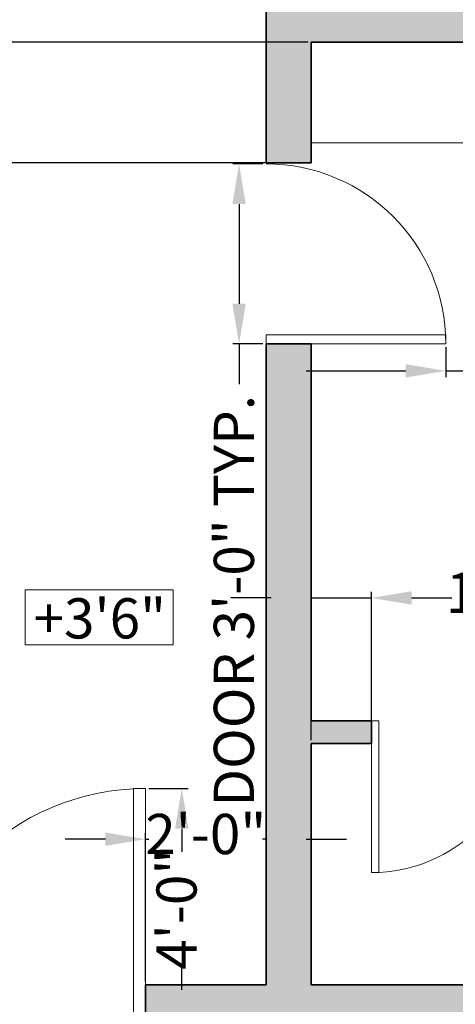
# Model space of a CAD drawing. Units: inches. Extents: x 2408 to 5087, y 2429 to 5085.
# Tile 8 of 12: x 2636 to 2723, y 2619 to 2815. Entities that reach past the tile are written whole.
import ezdxf

# ---------------------------------------------------------------- set-up
doc = ezdxf.new("R2010")
doc.units = ezdxf.units.IN
for name, color, linetype, lineweight in [('A-ANNO-DIMS', 2, 'Continuous', 18), ('A-ANNO-SYMB', 6, 'Continuous', 18), ('A-DOOR', 3, 'Continuous', 18), ('A-FLOR-CASE', 8, 'Continuous', 18), ('A-WALL', 7, 'Continuous', 35), ('A-WALL-PATT', 252, 'Continuous', 13)]:
    doc.layers.add(name, color=color, linetype=linetype, lineweight=lineweight)
doc.styles.get("Standard").update_dxf_attribs({"font": 'arial.ttf'})
doc.dimstyles.new('ISO-25', dxfattribs={"dimtxt": 8, "dimasz": 8, "dimexe": 1.25, "dimexo": 0.625, "dimtad": 0, "dimdec": 1, "dimlunit": 4, "dimtxsty": 'Standard', "dimcen": 2.5, "dimadec": 0, "dimazin": 0, "dimtfac": 1, "dimtdec": 1, "dimtmove": 0, "dimatfit": 3, "dimfxl": 1, "dimarcsym": 0})

# ---------------------------------------------------------------- blocks, each defined once
blk = doc.blocks.new('door')
blk.add_lwpolyline([(2353.25, 2862.23), (2353.25, 2898.06), (2351.47, 2898.06), (2351.47, 2862.23), (2353.25, 2862.23)])
blk.add_arc((2353.25, 2862.23), 35.83, 90, 180)
blk = doc.blocks.new('LEVEL-TAG-FRAME')
blk.add_line((29.47, 11), (29.47, 0))
blk.add_lwpolyline([(29.47, 0), (0, 0), (0, 11), (29.47, 11)])
blk = doc.blocks.new('*D27')
at = {"layer": 'A-ANNO-DIMS', "color": 0, "lineweight": -2, "transparency": 16777216}
for p, q in [((2612.36, 2568.68), (2612.36, 2576.68)), ((2608.98, 2568.68), (2613.61, 2568.68)), ((2612.36, 2550.04), (2612.36, 2560.68)), ((2608.98, 2542.04), (2613.61, 2542.04))]:
    blk.add_line(p, q, dxfattribs=at)
at = {"layer": 'A-ANNO-DIMS', "color": 0, "transparency": 16777216}
for points in [[(2611.02, 2560.68), (2613.69, 2560.68), (2612.36, 2568.68)], [(2611.02, 2550.04), (2613.69, 2550.04), (2612.36, 2542.04)]]:
    blk.add_solid(points, dxfattribs=at)
at = {"layer": 'Defpoints', "color": 0, "transparency": 16777216}
for p in [(2608.36, 2568.68), (2612.36, 2568.68), (2608.36, 2542.04)]:
    blk.add_point(p, dxfattribs=at)
at = {"layer": 'A-ANNO-DIMS', "color": 0, "transparency": 16777216, "insert": (2612.36, 2631.3), "char_height": 8, "attachment_point": 5, "rotation": 90}
blk.add_mtext('PAVER 2\'-2 1/2" TYP.', dxfattribs=at)
blk = doc.blocks.new('*D37')
at = {"layer": 'A-ANNO-DIMS', "color": 0, "lineweight": -2, "transparency": 16777216}
for p, q in [((2684.87, 2785.87), (2678.87, 2785.87)), ((2680.12, 2777.87), (2680.12, 2758.05)), ((2684.87, 2750.05), (2678.87, 2750.05)), ((2680.12, 2750.05), (2680.12, 2742.05))]:
    blk.add_line(p, q, dxfattribs=at)
at = {"layer": 'A-ANNO-DIMS', "color": 0, "transparency": 16777216}
for points in [[(2678.79, 2777.87), (2681.45, 2777.87), (2680.12, 2785.87)], [(2678.79, 2758.05), (2681.45, 2758.05), (2680.12, 2750.05)]]:
    blk.add_solid(points, dxfattribs=at)
at = {"layer": 'Defpoints', "color": 0, "transparency": 16777216}
for p in [(2685.49, 2785.87), (2680.12, 2750.05), (2685.49, 2750.05)]:
    blk.add_point(p, dxfattribs=at)
at = {"layer": 'A-ANNO-DIMS', "color": 0, "transparency": 16777216, "insert": (2680.12, 2698.93), "char_height": 8, "attachment_point": 5, "rotation": 90}
blk.add_mtext('DOOR 3\'-0" TYP.', dxfattribs=at)
blk = doc.blocks.new('*D38')
at = {"layer": 'A-ANNO-DIMS', "color": 0, "lineweight": -2, "transparency": 16777216}
for p, q in [((2685.49, 2749.43), (2685.49, 2743.43)), ((2721.31, 2749.43), (2721.31, 2743.43)), ((2693.49, 2744.68), (2713.31, 2744.68)), ((2721.31, 2744.68), (2729.31, 2744.68))]:
    blk.add_line(p, q, dxfattribs=at)
at = {"layer": 'A-ANNO-DIMS', "color": 0, "transparency": 16777216}
for points in [[(2693.49, 2746.02), (2693.49, 2743.35), (2685.49, 2744.68)], [(2713.31, 2746.02), (2713.31, 2743.35), (2721.31, 2744.68)]]:
    blk.add_solid(points, dxfattribs=at)
at = {"layer": 'Defpoints', "color": 0, "transparency": 16777216}
for p in [(2685.49, 2750.05), (2721.31, 2750.05), (2721.31, 2744.68)]:
    blk.add_point(p, dxfattribs=at)
at = {"layer": 'A-ANNO-DIMS', "color": 0, "transparency": 16777216, "insert": (2754.31, 2744.68), "char_height": 8, "attachment_point": 5}
blk.add_mtext('3\'-0" TYP.', dxfattribs=at)
blk = doc.blocks.new('*D40')
at = {"layer": 'A-ANNO-DIMS', "color": 0, "lineweight": -2, "transparency": 16777216}
for p, q in [((2662.12, 2661.59), (2669.95, 2661.59)), ((2668.7, 2653.59), (2668.7, 2648.99)), ((2668.7, 2621.55), (2668.7, 2626.15)), ((2662.12, 2613.55), (2669.95, 2613.55))]:
    blk.add_line(p, q, dxfattribs=at)
at = {"layer": 'A-ANNO-DIMS', "color": 0, "transparency": 16777216}
for points in [[(2667.37, 2653.59), (2670.03, 2653.59), (2668.7, 2661.59)], [(2667.37, 2621.55), (2670.03, 2621.55), (2668.7, 2613.55)]]:
    blk.add_solid(points, dxfattribs=at)
at = {"layer": 'Defpoints', "color": 0, "transparency": 16777216}
for p in [(2661.49, 2661.59), (2668.7, 2661.59), (2661.49, 2613.55)]:
    blk.add_point(p, dxfattribs=at)
at = {"layer": 'A-ANNO-DIMS', "color": 0, "transparency": 16777216, "insert": (2668.7, 2637.57), "char_height": 8, "attachment_point": 5, "rotation": 90}
blk.add_mtext('4\'-0"', dxfattribs=at)
blk = doc.blocks.new('*D75')
at = {"layer": 'A-ANNO-DIMS', "color": 0, "lineweight": -2, "transparency": 16777216}
for p, q in [((2661.49, 2623.18), (2661.49, 2652.75)), ((2685.49, 2623.18), (2685.49, 2652.75)), ((2653.49, 2651.5), (2645.49, 2651.5)), ((2661.49, 2651.5), (2662.17, 2651.5)), ((2685.49, 2651.5), (2684.82, 2651.5)), ((2693.49, 2651.5), (2701.49, 2651.5))]:
    blk.add_line(p, q, dxfattribs=at)
at = {"layer": 'A-ANNO-DIMS', "color": 0, "transparency": 16777216}
for points in [[(2653.49, 2652.84), (2653.49, 2650.17), (2661.49, 2651.5)], [(2693.49, 2652.84), (2693.49, 2650.17), (2685.49, 2651.5)]]:
    blk.add_solid(points, dxfattribs=at)
at = {"layer": 'Defpoints', "color": 0, "transparency": 16777216}
for p in [(2685.49, 2651.5), (2661.49, 2622.55), (2685.49, 2622.55)]:
    blk.add_point(p, dxfattribs=at)
at = {"layer": 'A-ANNO-DIMS', "color": 0, "transparency": 16777216, "insert": (2673.49, 2651.5), "char_height": 8, "attachment_point": 5}
blk.add_mtext('2\'-0"', dxfattribs=at)
blk = doc.blocks.new('*D79')
at = {"layer": 'A-ANNO-DIMS', "color": 0, "lineweight": -2, "transparency": 16777216}
for p, q in [((2432.93, 2818.05), (2432.93, 2826.05)), ((2693.87, 2810.05), (2431.68, 2810.05)), ((2432.93, 2810.05), (2432.93, 2809.38)), ((2693.87, 2786.05), (2431.68, 2786.05)), ((2432.93, 2786.05), (2432.93, 2786.73)), ((2432.93, 2778.05), (2432.93, 2770.05))]:
    blk.add_line(p, q, dxfattribs=at)
at = {"layer": 'A-ANNO-DIMS', "color": 0, "transparency": 16777216}
for points in [[(2431.59, 2818.05), (2434.26, 2818.05), (2432.93, 2810.05)], [(2431.59, 2778.05), (2434.26, 2778.05), (2432.93, 2786.05)]]:
    blk.add_solid(points, dxfattribs=at)
at = {"layer": 'Defpoints', "color": 0, "transparency": 16777216}
for p in [(2432.93, 2810.05), (2694.49, 2810.05), (2694.49, 2786.05)]:
    blk.add_point(p, dxfattribs=at)
at = {"layer": 'A-ANNO-DIMS', "color": 0, "transparency": 16777216, "insert": (2432.93, 2798.05), "char_height": 8, "attachment_point": 5, "rotation": 90}
blk.add_mtext('2\'-0"', dxfattribs=at)
blk = doc.blocks.new('*D80')
at = {"layer": 'A-ANNO-DIMS', "color": 0, "lineweight": -2, "transparency": 16777216}
for p, q in [((2694.49, 2671.18), (2694.49, 2700.75)), ((2706.49, 2671.18), (2706.49, 2700.75)), ((2686.49, 2699.5), (2678.49, 2699.5)), ((2694.49, 2699.5), (2706.49, 2699.5)), ((2714.49, 2699.5), (2722.49, 2699.5))]:
    blk.add_line(p, q, dxfattribs=at)
at = {"layer": 'A-ANNO-DIMS', "color": 0, "transparency": 16777216}
for points in [[(2686.49, 2700.84), (2686.49, 2698.17), (2694.49, 2699.5)], [(2714.49, 2700.84), (2714.49, 2698.17), (2706.49, 2699.5)]]:
    blk.add_solid(points, dxfattribs=at)
at = {"layer": 'Defpoints', "color": 0, "transparency": 16777216}
for p in [(2706.49, 2699.5), (2694.49, 2670.55), (2706.49, 2670.55)]:
    blk.add_point(p, dxfattribs=at)
at = {"layer": 'A-ANNO-DIMS', "color": 0, "transparency": 16777216, "insert": (2733.38, 2699.5), "char_height": 8, "attachment_point": 5}
blk.add_mtext('1\'-0"', dxfattribs=at)

msp = doc.modelspace()

# ---------------------------------------------------------------- hatches: boundary and pattern name
at = {"layer": 'A-WALL-PATT'}
h = msp.add_hatch(color=256, dxfattribs=at)
h.dxf.hatch_style = 1
h.paths.add_polyline_path([(2493.49, 2613.55), (2523.49, 2613.55), (2523.49, 2622.55), (2493.49, 2622.55), (2493.49, 2714.8), (2484.49, 2714.8), (2484.49, 2497.75), (2493.49, 2497.75)])
h.paths.add_polyline_path([(2613.49, 2615.42), (2613.49, 2622.55), (2583.49, 2622.55), (2583.49, 2613.55), (2613.46, 2613.55, -0.009707)])
h.paths.add_polyline_path([(2823.49, 2634.55), (2814.49, 2634.55), (2814.49, 2622.55), (2694.49, 2622.55), (2694.49, 2670.55), (2706.49, 2670.55), (2706.49, 2675.05), (2694.49, 2675.05), (2694.49, 2750.05), (2685.49, 2750.05), (2685.49, 2622.55), (2661.49, 2622.55), (2661.49, 2613.55), (2814.49, 2613.55), (2814.49, 2522.05), (2688.49, 2522.05), (2688.49, 2513.05), (2823.49, 2513.05)])
h.paths.add_polyline_path([(2823.49, 2837.05), (2814.49, 2837.05), (2814.49, 2819.05), (2685.49, 2819.05), (2685.49, 2786.05), (2694.49, 2786.05), (2694.49, 2810.05), (2814.49, 2810.05), (2814.49, 2772.55), (2823.49, 2772.55)])
h.paths.add_polyline_path([(2694.49, 2964.55), (2595.49, 2964.55), (2595.49, 3008.05), (2601.49, 3008.05), (2601.49, 3017.05), (2484.49, 3017.05), (2484.49, 2972.05), (2493.49, 2972.05), (2493.49, 3008.05), (2586.49, 3008.05), (2586.49, 2955.55), (2685.49, 2955.55), (2685.49, 2854.87), (2694.49, 2854.87)])
h.paths.add_polyline_path([(2493.49, 2867.05), (2595.49, 2867.05), (2595.49, 2876.05), (2493.49, 2876.05), (2493.49, 2912.05), (2484.49, 2912.05), (2484.49, 2774.8), (2493.49, 2774.8)])
h.paths.add_polyline_path([(2595.49, 2814.55), (2493.49, 2814.55), (2493.49, 2810.05), (2595.49, 2810.05)], flags=17)
h.paths.add_polyline_path([(2724.49, 3017.05), (2625.49, 3017.05), (2625.49, 3008.05), (2685.49, 3008.05), (2685.49, 2994.55), (2694.49, 2994.55), (2694.49, 3008.05), (2724.49, 3008.05)])
h.paths.add_polyline_path([(2823.49, 3017.05), (2784.49, 3017.05), (2784.49, 3008.05), (2814.49, 3008.05), (2814.49, 2913.55), (2814.56, 2897.05), (2823.49, 2897.05)])
h.paths.add_polyline_path([(2823.49, 2712.55), (2814.61, 2712.55), (2814.66, 2701.27), (2814.49, 2701.27), (2814.49, 2675.05), (2740.99, 2675.05), (2740.99, 2687.05), (2736.49, 2687.05), (2736.49, 2670.55), (2814.49, 2670.55), (2814.49, 2658.55), (2823.49, 2658.55)], flags=17)

# ---------------------------------------------------------------- linework, layer by layer
at = {"layer": 'A-FLOR-CASE'}
msp.add_line((2814.49, 2790.05), (2694.49, 2790.05), dxfattribs=at)
at = {"layer": 'A-WALL'}
for p, q in [((2685.49, 2819.05), (2685.49, 2786.05)), ((2814.49, 2810.05), (2694.49, 2810.05)), ((2694.49, 2810.05), (2694.49, 2786.05)), ((2694.49, 2786.05), (2685.49, 2786.05)), ((2694.49, 2750.05), (2685.49, 2750.05)), ((2685.49, 2750.05), (2685.49, 2622.55)), ((2694.49, 2750.05), (2694.49, 2675.05)), ((2706.49, 2675.05), (2694.49, 2675.05)), ((2706.49, 2675.05), (2706.49, 2670.55)), ((2706.49, 2670.55), (2694.49, 2670.55)), ((2694.49, 2670.55), (2694.49, 2622.55)), ((2661.49, 2622.55), (2661.49, 2613.55)), ((2685.49, 2622.55), (2661.49, 2622.55)), ((2814.49, 2622.55), (2694.49, 2622.55))]:
    msp.add_line(p, q, dxfattribs=at)

# ---------------------------------------------------------------- block references
at = {"layer": 'A-ANNO-SYMB'}
msp.add_blockref('LEVEL-TAG-FRAME', (2637.52, 2690.15), dxfattribs=at)
at = {"layer": 'A-DOOR'}
for p, xscale, yscale, zscale, rotation in [((-175.85, 5102.56), 0.9996876399039416, 0.9996876399039416, 0.9996876399039416, 270), ((4689.44, 5086.9), 0.8426439767912587, 0.8426439767912587, 0.8426439767912587, 180)]:
    msp.add_blockref('door', p, dxfattribs=dict(at, xscale=xscale, yscale=yscale, zscale=zscale, rotation=rotation))
at = {"layer": 'A-DOOR', "xscale": 1.340790722123845, "yscale": 1.340790722123845, "zscale": 1.340790722123845}
msp.add_blockref('door', (-493.72, -1224.1), dxfattribs=at)

# ---------------------------------------------------------------- texts
at = {"layer": 'A-ANNO-SYMB', "insert": (2600.95, 2699.44), "char_height": 8, "attachment_point": 1}
msp.add_mtext_dynamic_manual_height_columns('\\pxqc;+3\'6"', width=102.8772, gutter_width=12.5, heights=[0], dxfattribs=at)

# ---------------------------------------------------------------- dimensions: what is measured, and where the dimension line sits
at = {"layer": 'A-ANNO-DIMS'}
for base, p1, p2, picture, middle in [((2432.93, 2810.05), (2694.49, 2786.05), (2694.49, 2810.05), '*D79', (2432.93, 2798.05)), ((2668.7, 2661.59), (2661.49, 2613.55), (2661.49, 2661.59), '*D40', (2668.7, 2637.57))]:
    dim = msp.add_linear_dim(base=base, p1=p1, p2=p2, angle=90, dimstyle='ISO-25', override={"dimdec": 1, "dimlfac": 1, "dimrnd": 0, "dimzin": 1, "dimdsep": 46, "dimlunit": 4, "dimfrac": 2}, dxfattribs=at)
    dim.commit()
    dim.dimension.update_dxf_attribs({"geometry": picture, "text_midpoint": middle})
for base, p1, p2, angle, text, picture, middle in [((2680.12, 2750.05), (2685.49, 2785.87), (2685.49, 2750.05), 270, 'DOOR <> TYP.', '*D37', (2680.12, 2698.93)), ((2612.36, 2568.68), (2608.36, 2542.04), (2608.36, 2568.68), 90, 'PAVER <> TYP.', '*D27', (2612.36, 2631.3))]:
    dim = msp.add_linear_dim(base=base, p1=p1, p2=p2, angle=angle, text=text, dimstyle='ISO-25', override={"dimdec": 1, "dimlfac": 1, "dimrnd": 0, "dimzin": 1, "dimdsep": 46, "dimlunit": 4, "dimfrac": 2}, dxfattribs=at)
    dim.commit()
    dim.dimension.update_dxf_attribs({"geometry": picture, "text_midpoint": middle})
dim = msp.add_linear_dim(base=(2721.31, 2744.68), p1=(2685.49, 2750.05), p2=(2721.31, 2750.05), text='<> TYP.', dimstyle='ISO-25', override={"dimdec": 1, "dimlfac": 1, "dimrnd": 0, "dimzin": 1, "dimdsep": 46, "dimlunit": 4, "dimfrac": 2}, dxfattribs=at)
dim.commit()
dim.dimension.update_dxf_attribs({"geometry": '*D38', "text_midpoint": (2754.31, 2744.68)})
for base, p1, p2, picture, middle in [((2706.49, 2699.5), (2694.49, 2670.55), (2706.49, 2670.55), '*D80', (2733.38, 2699.5)), ((2685.49, 2651.5), (2661.49, 2622.55), (2685.49, 2622.55), '*D75', (2673.49, 2651.5))]:
    dim = msp.add_linear_dim(base=base, p1=p1, p2=p2, dimstyle='ISO-25', override={"dimdec": 1, "dimlfac": 1, "dimrnd": 0, "dimzin": 1, "dimdsep": 46, "dimlunit": 4, "dimfrac": 2}, dxfattribs=at)
    dim.commit()
    dim.dimension.update_dxf_attribs({"geometry": picture, "text_midpoint": middle})

doc.saveas('drawing.dxf')
